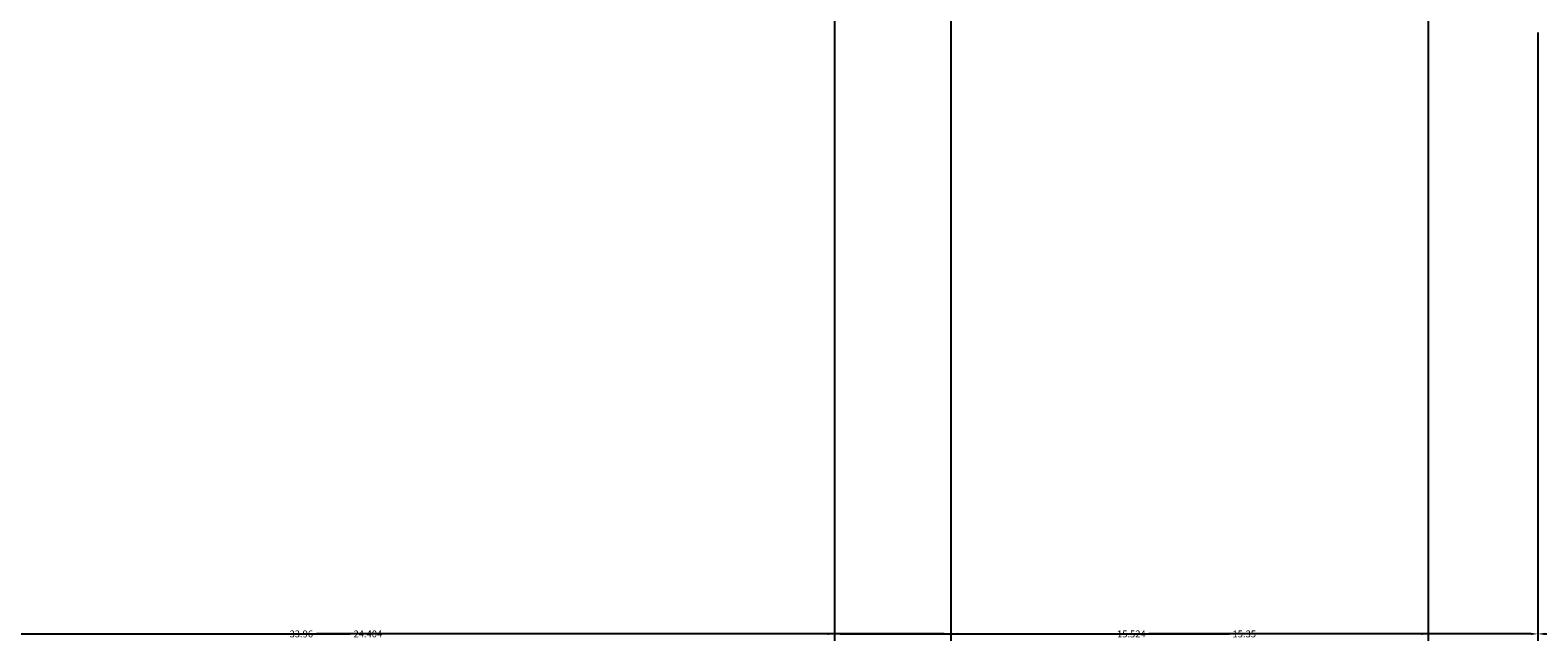
# Model space of a CAD drawing. Units: feet. Extents: x 2695 to 2912, y 795 to 1139.
# Tile 3 of 83: x 2734 to 2774, y 795 to 811. Entities that reach past the tile are written whole.
import ezdxf

# ---------------------------------------------------------------- set-up
doc = ezdxf.new("R2010")
doc.units = ezdxf.units.FT
doc.layers.add('A-ANNO-DIMS', color=2, linetype='Continuous', lineweight=18)
doc.styles.get("Standard").update_dxf_attribs({"font": 'arial.ttf'})
doc.dimstyles.get("Standard").update_dxf_attribs({"dimtxt": 0.18, "dimasz": 0.18, "dimexe": 0.18, "dimexo": 0.0625, "dimgap": 0.09, "dimtad": 0, "dimtih": 1, "dimtoh": 1, "dimdec": 1, "dimzin": 0, "dimdsep": 46, "dimlunit": 3, "dimtxsty": 'Standard', "dimcen": 0.09, "dimadec": 0, "dimazin": 0, "dimtfac": 1, "dimtdec": 1, "dimtofl": 0, "dimtmove": 0, "dimatfit": 3, "dimfxl": 1, "dimtolj": 1, "dimtzin": 0, "dimarcsym": 0})

# ---------------------------------------------------------------- blocks, each defined once
blk = doc.blocks.new('*D3')
at = {"layer": 'A-ANNO-DIMS', "color": 0, "lineweight": -2, "transparency": 16777216}
for p, q in [((2724.189, 874.795), (2724.189, 794.976)), ((2758.151, 874.795), (2758.151, 794.976)), ((2724.369, 795.156), (2740.777, 795.156)), ((2757.971, 795.156), (2741.564, 795.156))]:
    blk.add_line(p, q, dxfattribs=at)
at = {"layer": 'A-ANNO-DIMS', "color": 0, "transparency": 16777216}
for points in [[(2724.369, 795.186), (2724.369, 795.126), (2724.189, 795.156)], [(2757.971, 795.186), (2757.971, 795.126), (2758.151, 795.156)]]:
    blk.add_solid(points, dxfattribs=at)
at = {"layer": 'Defpoints', "color": 0, "transparency": 16777216}
for p in [(2724.189, 874.857), (2758.151, 874.857), (2758.151, 795.156)]:
    blk.add_point(p, dxfattribs=at)
at = {"layer": 'A-ANNO-DIMS', "color": 0, "transparency": 16777216, "insert": (2741.17, 795.156), "char_height": 0.18, "attachment_point": 5}
blk.add_mtext('\\A1;33.96', dxfattribs=at)
blk = doc.blocks.new('*D4')
at = {"layer": 'A-ANNO-DIMS', "color": 0, "lineweight": -2, "transparency": 16777216}
for p, q in [((2758.151, 874.795), (2758.151, 794.976)), ((2773.503, 810.868), (2773.503, 794.976)), ((2758.331, 795.156), (2765.441, 795.156)), ((2773.323, 795.156), (2766.213, 795.156))]:
    blk.add_line(p, q, dxfattribs=at)
at = {"layer": 'A-ANNO-DIMS', "color": 0, "transparency": 16777216}
for points in [[(2758.331, 795.186), (2758.331, 795.126), (2758.151, 795.156)], [(2773.323, 795.186), (2773.323, 795.126), (2773.503, 795.156)]]:
    blk.add_solid(points, dxfattribs=at)
at = {"layer": 'Defpoints', "color": 0, "transparency": 16777216}
for p in [(2758.151, 874.857), (2773.503, 810.931), (2773.503, 795.156)]:
    blk.add_point(p, dxfattribs=at)
at = {"layer": 'A-ANNO-DIMS', "color": 0, "transparency": 16777216, "insert": (2765.827, 795.156), "char_height": 0.18, "attachment_point": 5}
blk.add_mtext('\\A1;15.35', dxfattribs=at)
blk = doc.blocks.new('*D5')
at = {"layer": 'A-ANNO-DIMS', "color": 0, "lineweight": -2, "transparency": 16777216}
for p, q in [((2773.503, 810.868), (2773.503, 794.976)), ((2838.377, 810.868), (2838.377, 794.976)), ((2773.683, 795.156), (2805.546, 795.156)), ((2838.197, 795.156), (2806.334, 795.156))]:
    blk.add_line(p, q, dxfattribs=at)
at = {"layer": 'A-ANNO-DIMS', "color": 0, "transparency": 16777216}
for points in [[(2773.683, 795.186), (2773.683, 795.126), (2773.503, 795.156)], [(2838.197, 795.186), (2838.197, 795.126), (2838.377, 795.156)]]:
    blk.add_solid(points, dxfattribs=at)
at = {"layer": 'Defpoints', "color": 0, "transparency": 16777216}
for p in [(2773.503, 810.931), (2838.377, 810.931), (2838.377, 795.156)]:
    blk.add_point(p, dxfattribs=at)
at = {"layer": 'A-ANNO-DIMS', "color": 0, "transparency": 16777216, "insert": (2805.94, 795.156), "char_height": 0.18, "attachment_point": 5}
blk.add_mtext('\\A1;64.87', dxfattribs=at)
blk = doc.blocks.new('*D13')
at = {"layer": 'A-ANNO-DIMS', "color": 0, "lineweight": -2, "transparency": 16777216}
for p, q in [((2758.214, 874.857), (2911.424, 874.857)), ((2911.244, 874.677), (2911.244, 843.076)), ((2911.244, 811.111), (2911.244, 842.712)), ((2890.699, 810.931), (2911.424, 810.931))]:
    blk.add_line(p, q, dxfattribs=at)
at = {"layer": 'A-ANNO-DIMS', "color": 0, "transparency": 16777216}
for points in [[(2911.214, 874.677), (2911.274, 874.677), (2911.244, 874.857)], [(2911.214, 811.111), (2911.274, 811.111), (2911.244, 810.931)]]:
    blk.add_solid(points, dxfattribs=at)
at = {"layer": 'Defpoints', "color": 0, "transparency": 16777216}
for p in [(2758.151, 874.857), (2911.244, 874.857), (2890.636, 810.931)]:
    blk.add_point(p, dxfattribs=at)
at = {"layer": 'A-ANNO-DIMS', "color": 0, "transparency": 16777216, "insert": (2911.244, 842.894), "char_height": 0.18, "attachment_point": 5}
blk.add_mtext('\\A1;63.93', dxfattribs=at)
blk = doc.blocks.new('*D24')
at = {"layer": 'A-ANNO-DIMS', "color": 0, "lineweight": -2, "transparency": 16777216}
for p, q in [((2730.708, 936.868), (2730.708, 794.976)), ((2755.112, 936.868), (2755.112, 794.976)), ((2730.888, 795.156), (2742.446, 795.156)), ((2754.932, 795.156), (2743.375, 795.156))]:
    blk.add_line(p, q, dxfattribs=at)
at = {"layer": 'A-ANNO-DIMS', "color": 0, "transparency": 16777216}
for points in [[(2730.888, 795.186), (2730.888, 795.126), (2730.708, 795.156)], [(2754.932, 795.186), (2754.932, 795.126), (2755.112, 795.156)]]:
    blk.add_solid(points, dxfattribs=at)
at = {"layer": 'Defpoints', "color": 0, "transparency": 16777216}
for p in [(2730.708, 936.931), (2755.112, 936.931), (2755.112, 795.156)]:
    blk.add_point(p, dxfattribs=at)
at = {"layer": 'A-ANNO-DIMS', "color": 0, "transparency": 16777216, "insert": (2742.91, 795.156), "char_height": 0.18, "attachment_point": 5}
blk.add_mtext('\\A1;24.404', dxfattribs=at)
blk = doc.blocks.new('*D25')
at = {"layer": 'A-ANNO-DIMS', "color": 0, "lineweight": -2, "transparency": 16777216}
for p, q in [((2755.112, 936.868), (2755.112, 794.976)), ((2770.636, 936.868), (2770.636, 794.976)), ((2755.292, 795.156), (2762.419, 795.156)), ((2770.456, 795.156), (2763.329, 795.156))]:
    blk.add_line(p, q, dxfattribs=at)
at = {"layer": 'A-ANNO-DIMS', "color": 0, "transparency": 16777216}
for points in [[(2755.292, 795.186), (2755.292, 795.126), (2755.112, 795.156)], [(2770.456, 795.186), (2770.456, 795.126), (2770.636, 795.156)]]:
    blk.add_solid(points, dxfattribs=at)
at = {"layer": 'Defpoints', "color": 0, "transparency": 16777216}
for p in [(2755.112, 936.931), (2770.636, 936.931), (2770.636, 795.156)]:
    blk.add_point(p, dxfattribs=at)
at = {"layer": 'A-ANNO-DIMS', "color": 0, "transparency": 16777216, "insert": (2762.874, 795.156), "char_height": 0.18, "attachment_point": 5}
blk.add_mtext('\\A1;15.524', dxfattribs=at)

msp = doc.modelspace()

# ---------------------------------------------------------------- dimensions: what is measured, and where the dimension line sits
at = {"layer": 'A-ANNO-DIMS'}
for base, p1, p2, override, picture, middle in [((2755.1125, 795.1556), (2730.7081, 936.9306), (2755.1125, 936.9306), {"dimdec": 3, "dimlfac": 1, "dimrnd": 0, "dimzin": 0, "dimdsep": 46, "dimlunit": 2}, '*D24', (2742.9103, 795.1556)), ((2770.6361, 795.1556), (2755.1125, 936.9306), (2770.6361, 936.9306), {"dimdec": 3, "dimlfac": 1, "dimrnd": 0, "dimzin": 0, "dimdsep": 46, "dimlunit": 2}, '*D25', (2762.8743, 795.1556)), ((2758.1515, 795.1556), (2724.1893, 874.8571), (2758.1515, 874.8571), {"dimdec": 2, "dimlfac": 1, "dimrnd": 0, "dimzin": 0, "dimdsep": 46, "dimlunit": 2}, '*D3', (2741.1704, 795.1556)), ((2773.5029, 795.1556), (2758.1515, 874.8571), (2773.5029, 810.9306), {"dimdec": 2, "dimlfac": 1, "dimrnd": 0, "dimzin": 0, "dimdsep": 46, "dimlunit": 2}, '*D4', (2765.8272, 795.1556)), ((2838.3767, 795.1556), (2773.5029, 810.9306), (2838.3767, 810.9306), {"dimdec": 2, "dimlfac": 1, "dimrnd": 0, "dimzin": 0, "dimdsep": 46, "dimlunit": 2}, '*D5', (2805.9398, 795.1556))]:
    dim = msp.add_linear_dim(base=base, p1=p1, p2=p2, dimstyle='Standard', override=override, dxfattribs=at)
    dim.commit()
    dim.dimension.update_dxf_attribs({"geometry": picture, "text_midpoint": middle})
dim = msp.add_linear_dim(base=(2911.2444, 874.8571), p1=(2890.6361, 810.9306), p2=(2758.1515, 874.8571), angle=90, dimstyle='Standard', override={"dimdec": 2, "dimlfac": 1, "dimrnd": 0, "dimzin": 0, "dimdsep": 46, "dimlunit": 2}, dxfattribs=at)
dim.commit()
dim.dimension.update_dxf_attribs({"geometry": '*D13', "text_midpoint": (2911.2444, 842.8938)})

doc.saveas('drawing.dxf')
